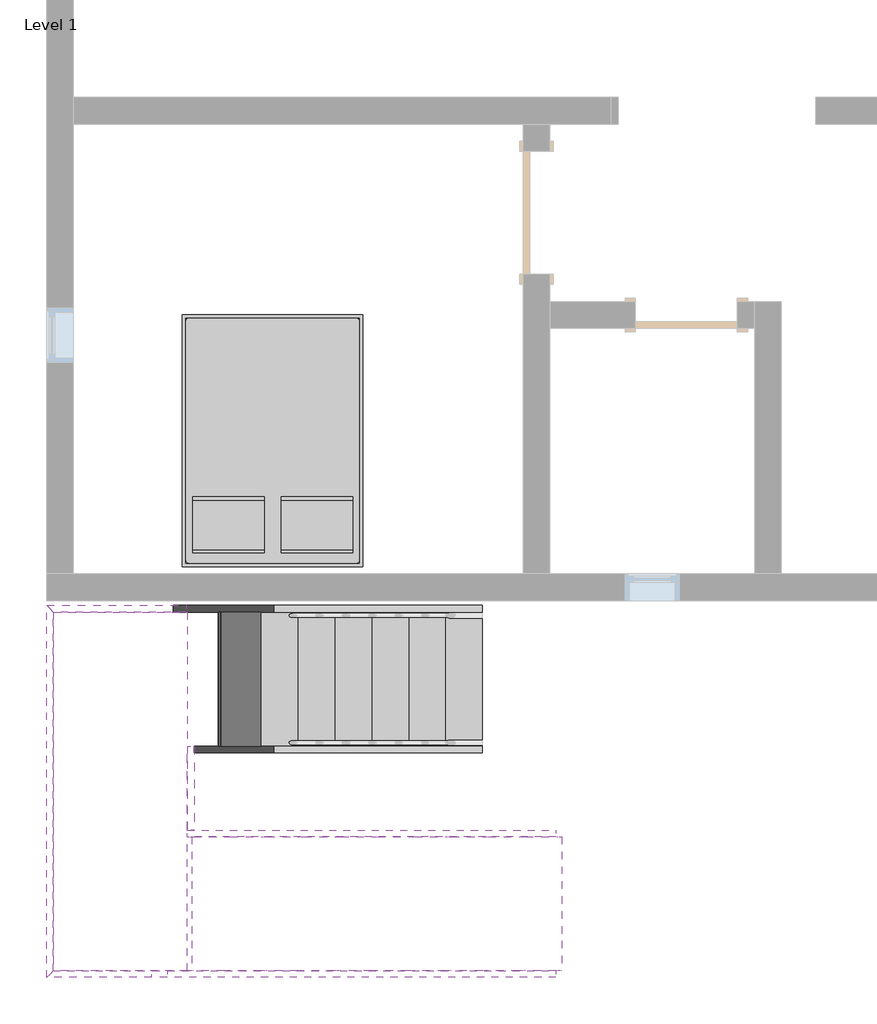
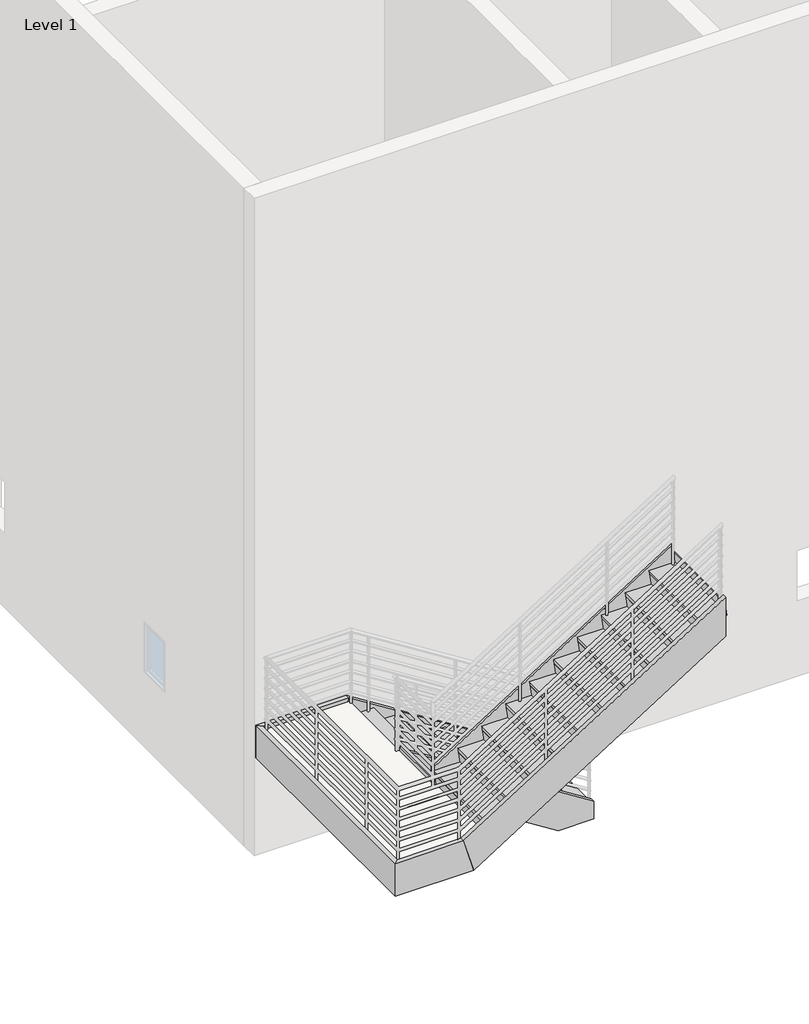
# One storey, part 4 of 4: 8 members, 2 stair flights, 1 furniture element, 1 slab.
"""IFC4 building model written with IfcOpenShell, lengths in millimetres."""

from ifc_helpers import new_model, si_unit, frame, origin, place, context, project, spatial, polyline, outline, extrude, faceted_brep, transform, mapped, element, save
from components import m_bed_box_1346_x_1880mm_double_b32eb57e, non_monolithic_landing_c0ded7b7, stair_flight_50mm_tread_25mm_nosing_13mm_riser_e6d86452, stair_flight_50mm_tread_25mm_nosing_13mm_riser_b2cb06da

model = new_model("IFC4")

# Units and contexts
model_context = context("Model", 3, world=origin())
ifc_project = project(units=[si_unit("LENGTHUNIT", "METRE", prefix="MILLI")], contexts=[model_context])

# Site, building, storey
site = spatial("IfcSite", under=ifc_project)
building = spatial("IfcBuilding", under=site)
storey = spatial("IfcBuildingStorey", under=building, Name="Level 1", Elevation=0.0)

# Furniture
placement = place(None, origin())
m_bed_box_1346_x_1880mm_double_shape = m_bed_box_1346_x_1880mm_double_b32eb57e(model_context)
element("IfcFurniture", 1, ObjectType="M_Bed-Box : 1346 x 1880mm - Double", at=placement, inside=storey, context=model_context, shape_type="MappedRepresentation", body=[
    mapped(m_bed_box_1346_x_1880mm_double_shape, transform((-9499.4968006, 7292.3138295, 0.0), x_axis=(-1.0, 0.0, 0.0), y_axis=(0.0, -1.0, 0.0), z_axis=(0.0, 0.0, 1.0))),
])

# Members
element("IfcMember", 2, ObjectType="Stringer - 50mm Width", at=placement, inside=storey, context=model_context, shape_type="SweptSolid", body=[
    extrude(outline(polyline([(0.0, -8274.8492596), (215.089535, -8274.8492596), (1574.7733295, -10424.8492596), (1101.4964536, -10424.8492596), (0.0, -8683.1079924), (0.0, -8274.8492596)])), frame((0.0, 5196.930447, 0.0), z_axis=(0.0, 1.0, 0.0), x_axis=(0.0, 0.0, 1.0)), (0.0, 0.0, 1.0), 50.0),
])
element("IfcMember", 3, ObjectType="Stringer - 50mm Width", at=placement, inside=storey, context=model_context, shape_type="SweptSolid", body=[
    extrude(outline(polyline([(0.0, -8274.8492596), (215.089535, -8274.8492596), (1612.6111183, -10484.6802631), (1212.6111183, -10600.5493232), (0.0, -8683.1079924), (0.0, -8274.8492596)])), frame((0.0, 6246.9562283, 0.0), z_axis=(0.0, 1.0, 0.0), x_axis=(0.0, 0.0, 1.0)), (0.0, 0.0, 1.0), 50.0),
])
element("IfcMember", 4, ObjectType="Stringer - 50mm Width", at=placement, inside=storey, context=model_context, shape_type="SweptSolid", body=[
    extrude(outline(polyline([(1780.3069263, -10474.8492596), (1307.0300504, -10474.8492596), (3046.1604852, -7724.8492596), (3519.4373611, -7724.8492596), (1780.3069263, -10474.8492596)])), frame((0.0, 4570.5562283, 0.0), z_axis=(0.0, 1.0, 0.0), x_axis=(0.0, 0.0, 1.0)), (0.0, 0.0, 1.0), 50.0),
])
element("IfcMember", 5, ObjectType="Stringer - 50mm Width", at=placement, inside=storey, context=model_context, shape_type="SweptSolid", body=[
    extrude(outline(polyline([(1612.6111183, -10740.0182561), (1212.6111183, -10624.149196), (3046.1604852, -7724.8492596), (3519.4373611, -7724.8492596), (1612.6111183, -10740.0182561)])), frame((0.0, 3520.530447, 0.0), z_axis=(0.0, 1.0, 0.0), x_axis=(0.0, 0.0, 1.0)), (0.0, 0.0, 1.0), 50.0),
])
element("IfcMember", 6, ObjectType="Stringer - 50mm Width", at=placement, inside=storey, context=model_context, shape_type="SweptSolid", body=[
    extrude(outline(polyline([(-10424.8492596, 4620.5562283), (-10474.8492596, 4620.5562283), (-10474.8492596, 5246.930447), (-10424.8492596, 5246.930447), (-10424.8492596, 4620.5562283)])), frame((0.0, 0.0, 1212.6111183), z_axis=(0.0, 0.0, 1.0), x_axis=(1.0, 0.0, 0.0)), (0.0, 0.0, 1.0), 400.0),
])
element("IfcMember", 7, ObjectType="Stringer - 50mm Width", at=placement, inside=storey, context=model_context, shape_type="Brep", body=[
    faceted_brep([(-10484.6802631, 6246.9562283, 1612.6111183), (-10484.6802631, 6296.9562283, 1612.6111183), (-11524.8750408, 6296.9562283, 1612.6111183), (-11474.8750408, 6246.9562283, 1612.6111183), (-10600.5493232, 6246.9562283, 1212.6111183), (-11474.8750408, 6246.9562283, 1212.6111183), (-10600.5493232, 6296.9562283, 1212.6111183), (-11524.8750408, 6296.9562283, 1212.6111183)], [[[0, 1, 2, 3]], [[4, 0, 3, 5]], [[6, 4, 5, 7]], [[1, 6, 7, 2]], [[1, 0, 4, 6]], [[2, 7, 5, 3]]]),
])
element("IfcMember", 8, ObjectType="Stringer - 50mm Width", at=placement, inside=storey, context=model_context, shape_type="SweptSolid", body=[
    extrude(outline(polyline([(-11524.8750408, 6296.9562283), (-11474.8750408, 6246.9562283), (-11474.8750408, 3570.530447), (-11524.8750408, 3520.530447), (-11524.8750408, 6296.9562283)])), frame((0.0, 0.0, 1212.6111183), z_axis=(0.0, 0.0, 1.0), x_axis=(1.0, 0.0, 0.0)), (0.0, 0.0, 1.0), 400.0),
])
element("IfcMember", 9, ObjectType="Stringer - 50mm Width", at=placement, inside=storey, context=model_context, shape_type="Brep", body=[
    faceted_brep([(-11474.8750408, 3570.530447, 1612.6111183), (-11524.8750408, 3520.530447, 1612.6111183), (-10740.0182561, 3520.530447, 1612.6111183), (-10740.0182561, 3570.530447, 1612.6111183), (-11474.8750408, 3570.530447, 1212.6111183), (-10624.149196, 3570.530447, 1212.6111183), (-11524.8750408, 3520.530447, 1212.6111183), (-10624.149196, 3520.530447, 1212.6111183)], [[[0, 1, 2, 3]], [[4, 0, 3, 5]], [[6, 4, 5, 7]], [[1, 6, 7, 2]], [[1, 0, 4, 6]], [[2, 7, 5, 3]]]),
])

# Slab
non_monolithic_landing_shape = non_monolithic_landing_c0ded7b7(model_context)
element("IfcSlab", 10, ObjectType="Non-Monolithic Landing", at=placement, inside=storey, context=model_context, shape_type="MappedRepresentation", body=[
    mapped(non_monolithic_landing_shape, transform((0.0, 0.0, 0.0), x_axis=(1.0, 0.0, 0.0), y_axis=(0.0, 1.0, 0.0), z_axis=(0.0, 0.0, 1.0))),
])

# Stair flights
stair_flight_50mm_tread_25mm_nosing_13mm_riser_shape = stair_flight_50mm_tread_25mm_nosing_13mm_riser_e6d86452(model_context)
element("IfcStairFlight", 11, ObjectType="50mm Tread 25mm Nosing 13mm Riser", at=placement, inside=storey, context=model_context, shape_type="MappedRepresentation", body=[
    mapped(stair_flight_50mm_tread_25mm_nosing_13mm_riser_shape, transform((0.0, 0.0, 0.0), x_axis=(1.0, 0.0, 0.0), y_axis=(0.0, 1.0, 0.0), z_axis=(0.0, 0.0, 1.0))),
])
stair_flight_50mm_tread_25mm_nosing_13mm_riser_2_shape = stair_flight_50mm_tread_25mm_nosing_13mm_riser_b2cb06da(model_context)
element("IfcStairFlight", 12, ObjectType="50mm Tread 25mm Nosing 13mm Riser", at=placement, inside=storey, context=model_context, shape_type="MappedRepresentation", body=[
    mapped(stair_flight_50mm_tread_25mm_nosing_13mm_riser_2_shape, transform((0.0, 0.0, 0.0), x_axis=(1.0, 0.0, 0.0), y_axis=(0.0, 1.0, 0.0), z_axis=(0.0, 0.0, 1.0))),
])

save(model, "model.ifc")

# Revit data of these elements
# Type "M_Bed-Box : 1346 x 1880mm - Double"
#   Length = 1880 mm
#   Width = 1346 mm
#   Frame Material = Birch
#   Mattress Material = Linen, White
#   Default Elevation = 0
# Element 1 (IfcFurniture, "M_Bed-Box : 1346 x 1880mm - Double")
#   Phase Created = New Construction
#   Materials on its faces: "Birch", "Linen, White"
# Elements 2, 3, 4, 5, 6, 7, 8, 9 (IfcMember, "Stringer - 50mm Width")
#   Phase Created = New Construction
# Element 10 (IfcSlab, "Non-Monolithic Landing")
#   Phase Created = New Construction
# Elements 11, 12 (IfcStairFlight, "50mm Tread 25mm Nosing 13mm Riser")
#   Phase Created = New Construction
# Materials
#   "Birch": class "Wood", colour RGB 224 178 126, transparency 0, Description = "Betula Alleghaniensis", Cost = 0
#   "Linen, White": class "Textile", colour RGB 247 247 239, transparency 0, Description = "Linen, white", Cost = 0
